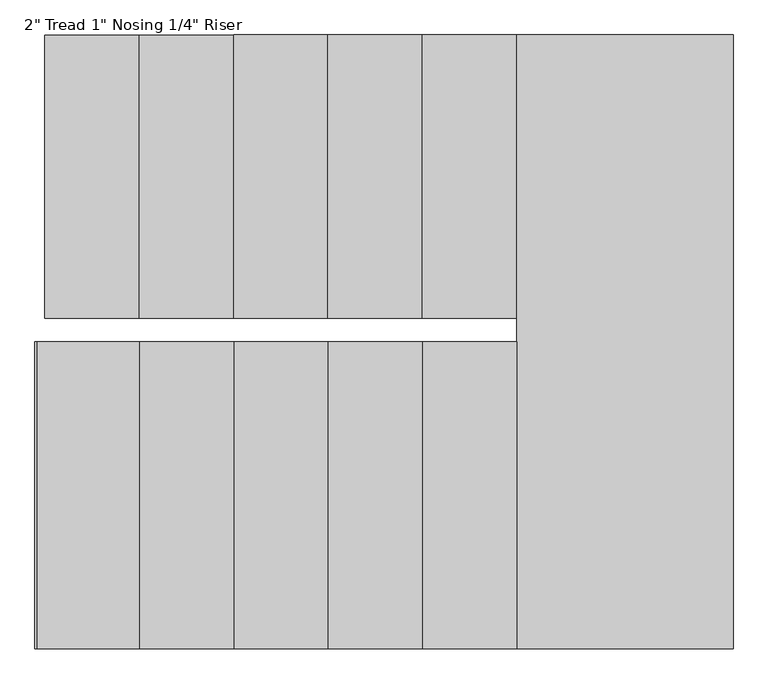
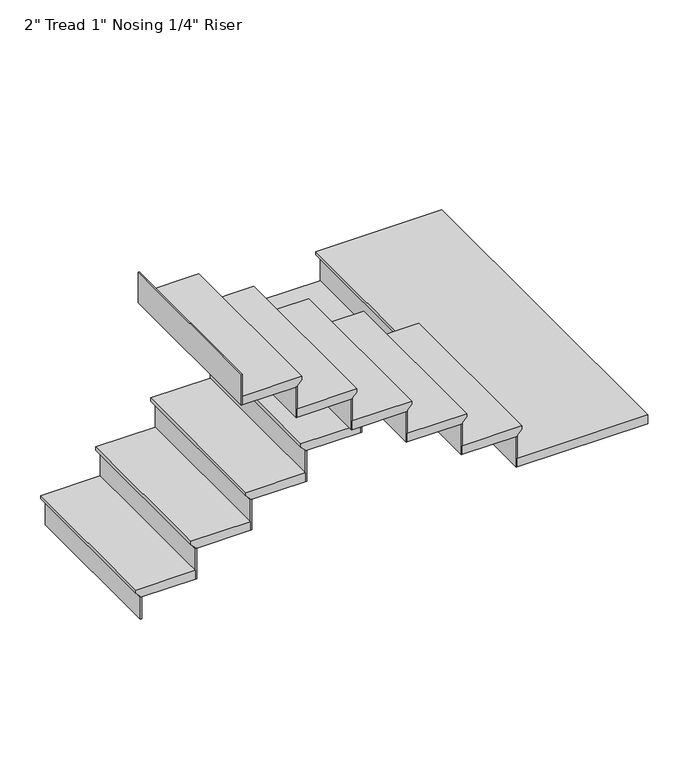
"""IFC4 building model written with IfcOpenShell, lengths in millimetres: stair flight geometry."""

from ifc_helpers import new_model, si_unit, origin, place, context, project, spatial, faceted_brep, source, transform, mapped, element, save


def stair_flight_ab8743af(model_context):
    return source(origin(), model_context, "Body", "Brep", [
        faceted_brep([(-1179.0415084, -2827.3064015, 160.2441176), (-1179.0415084, -2827.3064015, 179.2941176), (-1179.0415084, -1912.9064015, 179.2941176), (-1179.0415084, -1912.9064015, 160.2441176), (-1153.6415084, -2827.3064015, 134.8441176), (-1153.6415084, -1912.9064015, 134.8441176), (-848.8415084, -2827.3064015, 179.2941176), (-848.8415084, -1912.9064015, 179.2941176), (-1153.6415084, -1912.9064015, 128.4941176), (-848.8415084, -1912.9064015, 128.4941176), (-848.8415084, -2827.3064015, 128.4941176), (-1153.6415084, -2827.3064015, 128.4941176)], [[[0, 1, 2, 3]], [[4, 0, 3, 5]], [[2, 1, 6, 7]], [[8, 9, 10, 11]], [[2, 7, 9, 8, 5, 3]], [[8, 11, 4, 5]], [[6, 1, 0, 4, 11, 10]], [[7, 6, 10, 9]]]),
        faceted_brep([(-1153.6415084, -2827.3064015, 128.4941176), (-1153.6415084, -2827.3064015, 0.0), (-1147.2915084, -2827.3064015, 0.0), (-1147.2915084, -2827.3064015, 128.4941176), (-1153.6415084, -1912.9064015, 128.4941176), (-1147.2915084, -1912.9064015, 128.4941176), (-1147.2915084, -1912.9064015, 0.0), (-1153.6415084, -1912.9064015, 0.0)], [[[0, 1, 2, 3]], [[4, 5, 6, 7]], [[1, 0, 4, 7]], [[2, 1, 7, 6]], [[3, 2, 6, 5]], [[0, 3, 5, 4]]]),
        faceted_brep([(-848.8415084, -2827.3064015, 307.7882353), (-848.8415084, -2827.3064015, 128.4941176), (-842.4915084, -2827.3064015, 128.4941176), (-842.4915084, -2827.3064015, 307.7882353), (-848.8415084, -1912.9064015, 307.7882353), (-842.4915084, -1912.9064015, 307.7882353), (-842.4915084, -1912.9064015, 128.4941176), (-848.8415084, -1912.9064015, 128.4941176)], [[[0, 1, 2, 3]], [[4, 5, 6, 7]], [[1, 0, 4, 7]], [[2, 1, 7, 6]], [[3, 2, 6, 5]], [[0, 3, 5, 4]]]),
        faceted_brep([(-874.2415084, -1912.9064015, 358.5882353), (-874.2415084, -2827.3064015, 358.5882353), (-544.0415084, -2827.3064015, 358.5882353), (-544.0415084, -1912.9064015, 358.5882353), (-848.8415084, -1912.9064015, 307.7882353), (-544.0415084, -1912.9064015, 307.7882353), (-544.0415084, -2827.3064015, 307.7882353), (-848.8415084, -2827.3064015, 307.7882353), (-848.8415084, -1912.9064015, 314.1382353), (-874.2415084, -1912.9064015, 339.5382353), (-848.8415084, -2827.3064015, 314.1382353), (-874.2415084, -2827.3064015, 339.5382353)], [[[0, 1, 2, 3]], [[4, 5, 6, 7]], [[0, 3, 5, 4, 8, 9]], [[4, 7, 10, 8]], [[2, 1, 11, 10, 7, 6]], [[3, 2, 6, 5]], [[11, 1, 0, 9]], [[10, 11, 9, 8]]]),
        faceted_brep([(-544.0415084, -2827.3064015, 487.0823529), (-544.0415084, -2827.3064015, 307.7882353), (-537.6915084, -2827.3064015, 307.7882353), (-537.6915084, -2827.3064015, 487.0823529), (-544.0415084, -1912.9064015, 487.0823529), (-537.6915084, -1912.9064015, 487.0823529), (-537.6915084, -1912.9064015, 307.7882353), (-544.0415084, -1912.9064015, 307.7882353)], [[[0, 1, 2, 3]], [[4, 5, 6, 7]], [[1, 0, 4, 7]], [[2, 1, 7, 6]], [[3, 2, 6, 5]], [[0, 3, 5, 4]]]),
        faceted_brep([(-569.4415084, -1912.9064015, 537.8823529), (-569.4415084, -2827.3064015, 537.8823529), (-239.2415084, -2827.3064015, 537.8823529), (-239.2415084, -1912.9064015, 537.8823529), (-544.0415084, -1912.9064015, 487.0823529), (-239.2415084, -1912.9064015, 487.0823529), (-239.2415084, -2827.3064015, 487.0823529), (-544.0415084, -2827.3064015, 487.0823529), (-544.0415084, -1912.9064015, 493.4323529), (-569.4415084, -1912.9064015, 518.8323529), (-544.0415084, -2827.3064015, 493.4323529), (-569.4415084, -2827.3064015, 518.8323529)], [[[0, 1, 2, 3]], [[4, 5, 6, 7]], [[0, 3, 5, 4, 8, 9]], [[4, 7, 10, 8]], [[2, 1, 11, 10, 7, 6]], [[3, 2, 6, 5]], [[11, 1, 0, 9]], [[10, 11, 9, 8]]]),
        faceted_brep([(-239.2415084, -2827.3064015, 666.3764706), (-239.2415084, -2827.3064015, 487.0823529), (-232.8915084, -2827.3064015, 487.0823529), (-232.8915084, -2827.3064015, 666.3764706), (-239.2415084, -1912.9064015, 666.3764706), (-232.8915084, -1912.9064015, 666.3764706), (-232.8915084, -1912.9064015, 487.0823529), (-239.2415084, -1912.9064015, 487.0823529)], [[[0, 1, 2, 3]], [[4, 5, 6, 7]], [[1, 0, 4, 7]], [[2, 1, 7, 6]], [[3, 2, 6, 5]], [[0, 3, 5, 4]]]),
        faceted_brep([(-264.6415084, -1912.9064015, 717.1764706), (-264.6415084, -2827.3064015, 717.1764706), (65.5584916, -2827.3064015, 717.1764706), (65.5584916, -1912.9064015, 717.1764706), (-239.2415084, -1912.9064015, 666.3764706), (65.5584916, -1912.9064015, 666.3764706), (65.5584916, -2827.3064015, 666.3764706), (-239.2415084, -2827.3064015, 666.3764706), (-239.2415084, -1912.9064015, 672.7264706), (-264.6415084, -1912.9064015, 698.1264706), (-239.2415084, -2827.3064015, 672.7264706), (-264.6415084, -2827.3064015, 698.1264706)], [[[0, 1, 2, 3]], [[4, 5, 6, 7]], [[0, 3, 5, 4, 8, 9]], [[4, 7, 10, 8]], [[2, 1, 11, 10, 7, 6]], [[3, 2, 6, 5]], [[11, 1, 0, 9]], [[10, 11, 9, 8]]]),
        faceted_brep([(65.5584916, -2827.3064015, 845.6705882), (65.5584916, -2827.3064015, 666.3764706), (71.9084916, -2827.3064015, 666.3764706), (71.9084916, -2827.3064015, 845.6705882), (65.5584916, -1912.9064015, 845.6705882), (71.9084916, -1912.9064015, 845.6705882), (71.9084916, -1912.9064015, 666.3764706), (65.5584916, -1912.9064015, 666.3764706)], [[[0, 1, 2, 3]], [[4, 5, 6, 7]], [[1, 0, 4, 7]], [[2, 1, 7, 6]], [[3, 2, 6, 5]], [[0, 3, 5, 4]]]),
        faceted_brep([(40.1584916, -1912.9064015, 896.4705882), (40.1584916, -2827.3064015, 896.4705882), (370.3584916, -2827.3064015, 896.4705882), (370.3584916, -1912.9064015, 896.4705882), (65.5584916, -1912.9064015, 845.6705882), (370.3584916, -1912.9064015, 845.6705882), (370.3584916, -2827.3064015, 845.6705882), (65.5584916, -2827.3064015, 845.6705882), (65.5584916, -1912.9064015, 852.0205882), (40.1584916, -1912.9064015, 877.4205882), (65.5584916, -2827.3064015, 852.0205882), (40.1584916, -2827.3064015, 877.4205882)], [[[0, 1, 2, 3]], [[4, 5, 6, 7]], [[0, 3, 5, 4, 8, 9]], [[4, 7, 10, 8]], [[2, 1, 11, 10, 7, 6]], [[3, 2, 6, 5]], [[11, 1, 0, 9]], [[10, 11, 9, 8]]]),
        faceted_brep([(370.3584916, -2827.3064015, 1024.9647059), (370.3584916, -2827.3064015, 845.6705882), (376.7084916, -2827.3064015, 845.6705882), (376.7084916, -2827.3064015, 1024.9647059), (370.3584916, -1912.9064015, 1024.9647059), (376.7084916, -1912.9064015, 1024.9647059), (376.7084916, -1912.9064015, 845.6705882), (370.3584916, -1912.9064015, 845.6705882)], [[[0, 1, 2, 3]], [[4, 5, 6, 7]], [[1, 0, 4, 7]], [[2, 1, 7, 6]], [[3, 2, 6, 5]], [[0, 3, 5, 4]]]),
        faceted_brep([(319.5584916, -3894.1064015, 1075.7647059), (1043.4584916, -3894.1064015, 1075.7647059), (1043.4584916, -1912.9064015, 1075.7647059), (344.9584916, -1912.9064015, 1075.7647059), (344.9584916, -2903.5064015, 1075.7647059), (319.5584916, -2903.5064015, 1075.7647059), (1043.4584916, -3894.1064015, 1024.9647059), (319.5584916, -3894.1064015, 1024.9647059), (319.5584916, -2903.5064015, 1024.9647059), (344.9584916, -2903.5064015, 1024.9647059), (344.9584916, -2827.3064015, 1024.9647059), (370.3584916, -2827.3064015, 1024.9647059), (370.3584916, -1912.9064015, 1024.9647059), (1043.4584916, -1912.9064015, 1024.9647059), (370.3584916, -1912.9064015, 1031.3147059), (344.9584916, -1912.9064015, 1056.7147059), (370.3584916, -2827.3064015, 1031.3147059), (344.9584916, -2827.3064015, 1056.7147059)], [[[0, 1, 2, 3, 4, 5]], [[6, 7, 8, 9, 10, 11, 12, 13]], [[1, 0, 7, 6]], [[2, 1, 6, 13]], [[3, 2, 13, 12, 14, 15]], [[12, 11, 16, 14]], [[11, 10, 17, 16]], [[4, 3, 15, 17, 10, 9]], [[5, 4, 9, 8]], [[0, 5, 8, 7]], [[15, 14, 16, 17]]]),
        faceted_brep([(319.5584916, -2903.5064015, 1204.2588235), (319.5584916, -2903.5064015, 1024.9647059), (313.2084916, -2903.5064015, 1024.9647059), (313.2084916, -2903.5064015, 1204.2588235), (319.5584916, -3894.1064015, 1204.2588235), (313.2084916, -3894.1064015, 1204.2588235), (313.2084916, -3894.1064015, 1024.9647059), (319.5584916, -3894.1064015, 1024.9647059)], [[[0, 1, 2, 3]], [[4, 5, 6, 7]], [[1, 0, 4, 7]], [[2, 1, 7, 6]], [[3, 2, 6, 5]], [[0, 3, 5, 4]]]),
        faceted_brep([(344.9584916, -3894.1064015, 1255.0588235), (344.9584916, -2903.5064015, 1255.0588235), (14.7584916, -2903.5064015, 1255.0588235), (14.7584916, -3894.1064015, 1255.0588235), (319.5584916, -3894.1064015, 1204.2588235), (14.7584916, -3894.1064015, 1204.2588235), (14.7584916, -2903.5064015, 1204.2588235), (319.5584916, -2903.5064015, 1204.2588235), (319.5584916, -3894.1064015, 1210.6088235), (344.9584916, -3894.1064015, 1236.0088235), (319.5584916, -2903.5064015, 1210.6088235), (344.9584916, -2903.5064015, 1236.0088235)], [[[0, 1, 2, 3]], [[4, 5, 6, 7]], [[0, 3, 5, 4, 8, 9]], [[4, 7, 10, 8]], [[2, 1, 11, 10, 7, 6]], [[3, 2, 6, 5]], [[11, 1, 0, 9]], [[10, 11, 9, 8]]]),
        faceted_brep([(14.7584916, -2903.5064015, 1383.5529412), (14.7584916, -2903.5064015, 1204.2588235), (8.4084916, -2903.5064015, 1204.2588235), (8.4084916, -2903.5064015, 1383.5529412), (14.7584916, -3894.1064015, 1383.5529412), (8.4084916, -3894.1064015, 1383.5529412), (8.4084916, -3894.1064015, 1204.2588235), (14.7584916, -3894.1064015, 1204.2588235)], [[[0, 1, 2, 3]], [[4, 5, 6, 7]], [[1, 0, 4, 7]], [[2, 1, 7, 6]], [[3, 2, 6, 5]], [[0, 3, 5, 4]]]),
        faceted_brep([(40.1584916, -3894.1064015, 1434.3529412), (40.1584916, -2903.5064015, 1434.3529412), (-290.0415084, -2903.5064015, 1434.3529412), (-290.0415084, -3894.1064015, 1434.3529412), (14.7584916, -3894.1064015, 1383.5529412), (-290.0415084, -3894.1064015, 1383.5529412), (-290.0415084, -2903.5064015, 1383.5529412), (14.7584916, -2903.5064015, 1383.5529412), (14.7584916, -3894.1064015, 1389.9029412), (40.1584916, -3894.1064015, 1415.3029412), (14.7584916, -2903.5064015, 1389.9029412), (40.1584916, -2903.5064015, 1415.3029412)], [[[0, 1, 2, 3]], [[4, 5, 6, 7]], [[0, 3, 5, 4, 8, 9]], [[4, 7, 10, 8]], [[2, 1, 11, 10, 7, 6]], [[3, 2, 6, 5]], [[11, 1, 0, 9]], [[10, 11, 9, 8]]]),
        faceted_brep([(-290.0415084, -2903.5064015, 1562.8470588), (-290.0415084, -2903.5064015, 1383.5529412), (-296.3915084, -2903.5064015, 1383.5529412), (-296.3915084, -2903.5064015, 1562.8470588), (-290.0415084, -3894.1064015, 1562.8470588), (-296.3915084, -3894.1064015, 1562.8470588), (-296.3915084, -3894.1064015, 1383.5529412), (-290.0415084, -3894.1064015, 1383.5529412)], [[[0, 1, 2, 3]], [[4, 5, 6, 7]], [[1, 0, 4, 7]], [[2, 1, 7, 6]], [[3, 2, 6, 5]], [[0, 3, 5, 4]]]),
        faceted_brep([(-264.6415084, -3894.1064015, 1613.6470588), (-264.6415084, -2903.5064015, 1613.6470588), (-594.8415084, -2903.5064015, 1613.6470588), (-594.8415084, -3894.1064015, 1613.6470588), (-290.0415084, -3894.1064015, 1562.8470588), (-594.8415084, -3894.1064015, 1562.8470588), (-594.8415084, -2903.5064015, 1562.8470588), (-290.0415084, -2903.5064015, 1562.8470588), (-290.0415084, -3894.1064015, 1569.1970588), (-264.6415084, -3894.1064015, 1594.5970588), (-290.0415084, -2903.5064015, 1569.1970588), (-264.6415084, -2903.5064015, 1594.5970588)], [[[0, 1, 2, 3]], [[4, 5, 6, 7]], [[0, 3, 5, 4, 8, 9]], [[4, 7, 10, 8]], [[2, 1, 11, 10, 7, 6]], [[3, 2, 6, 5]], [[11, 1, 0, 9]], [[10, 11, 9, 8]]]),
        faceted_brep([(-594.8415084, -2903.5064015, 1742.1411765), (-594.8415084, -2903.5064015, 1562.8470588), (-601.1915084, -2903.5064015, 1562.8470588), (-601.1915084, -2903.5064015, 1742.1411765), (-594.8415084, -3894.1064015, 1742.1411765), (-601.1915084, -3894.1064015, 1742.1411765), (-601.1915084, -3894.1064015, 1562.8470588), (-594.8415084, -3894.1064015, 1562.8470588)], [[[0, 1, 2, 3]], [[4, 5, 6, 7]], [[1, 0, 4, 7]], [[2, 1, 7, 6]], [[3, 2, 6, 5]], [[0, 3, 5, 4]]]),
        faceted_brep([(-569.4415084, -3894.1064015, 1792.9411765), (-569.4415084, -2903.5064015, 1792.9411765), (-899.6415084, -2903.5064015, 1792.9411765), (-899.6415084, -3894.1064015, 1792.9411765), (-594.8415084, -3894.1064015, 1742.1411765), (-899.6415084, -3894.1064015, 1742.1411765), (-899.6415084, -2903.5064015, 1742.1411765), (-594.8415084, -2903.5064015, 1742.1411765), (-594.8415084, -3894.1064015, 1748.4911765), (-569.4415084, -3894.1064015, 1773.8911765), (-594.8415084, -2903.5064015, 1748.4911765), (-569.4415084, -2903.5064015, 1773.8911765)], [[[0, 1, 2, 3]], [[4, 5, 6, 7]], [[0, 3, 5, 4, 8, 9]], [[4, 7, 10, 8]], [[2, 1, 11, 10, 7, 6]], [[3, 2, 6, 5]], [[11, 1, 0, 9]], [[10, 11, 9, 8]]]),
        faceted_brep([(-899.6415084, -2903.5064015, 1921.4352941), (-899.6415084, -2903.5064015, 1742.1411765), (-905.9915084, -2903.5064015, 1742.1411765), (-905.9915084, -2903.5064015, 1921.4352941), (-899.6415084, -3894.1064015, 1921.4352941), (-905.9915084, -3894.1064015, 1921.4352941), (-905.9915084, -3894.1064015, 1742.1411765), (-899.6415084, -3894.1064015, 1742.1411765)], [[[0, 1, 2, 3]], [[4, 5, 6, 7]], [[1, 0, 4, 7]], [[2, 1, 7, 6]], [[3, 2, 6, 5]], [[0, 3, 5, 4]]]),
        faceted_brep([(-1204.4415084, -2903.5064015, 2100.7294118), (-1204.4415084, -2903.5064015, 1921.4352941), (-1210.7915084, -2903.5064015, 1921.4352941), (-1210.7915084, -2903.5064015, 2100.7294118), (-1204.4415084, -3894.1064015, 2100.7294118), (-1210.7915084, -3894.1064015, 2100.7294118), (-1210.7915084, -3894.1064015, 1921.4352941), (-1204.4415084, -3894.1064015, 1921.4352941)], [[[0, 1, 2, 3]], [[4, 5, 6, 7]], [[1, 0, 4, 7]], [[2, 1, 7, 6]], [[3, 2, 6, 5]], [[0, 3, 5, 4]]]),
        faceted_brep([(-874.2415084, -3894.1064015, 1972.2352941), (-874.2415084, -2903.5064015, 1972.2352941), (-1204.4415084, -2903.5064015, 1972.2352941), (-1204.4415084, -3894.1064015, 1972.2352941), (-899.6415084, -3894.1064015, 1921.4352941), (-1204.4415084, -3894.1064015, 1921.4352941), (-1204.4415084, -2903.5064015, 1921.4352941), (-899.6415084, -2903.5064015, 1921.4352941), (-899.6415084, -3894.1064015, 1927.7852941), (-874.2415084, -3894.1064015, 1953.1852941), (-899.6415084, -2903.5064015, 1927.7852941), (-874.2415084, -2903.5064015, 1953.1852941)], [[[0, 1, 2, 3]], [[4, 5, 6, 7]], [[0, 3, 5, 4, 8, 9]], [[4, 7, 10, 8]], [[2, 1, 11, 10, 7, 6]], [[3, 2, 6, 5]], [[11, 1, 0, 9]], [[10, 11, 9, 8]]]),
    ])


if __name__ == "__main__":
    model = new_model("IFC4")
    model_context = context("Model", 3, world=origin())
    ifc_project = project(units=[si_unit("LENGTHUNIT", "METRE", prefix="MILLI")], contexts=[model_context])
    site = spatial("IfcSite", under=ifc_project)
    building = spatial("IfcBuilding", under=site)
    placement = place(None, origin())
    stair_flight_shape = stair_flight_ab8743af(model_context)
    element("IfcStairFlight", 1, ObjectType="2\" Tread 1\" Nosing 1/4\" Riser", at=placement, inside=building, context=model_context, shape_type="MappedRepresentation", body=[
        mapped(stair_flight_shape, transform((0.0, 0.0, 0.0), x_axis=(1.0, 0.0, 0.0), y_axis=(0.0, 1.0, 0.0), z_axis=(0.0, 0.0, 1.0))),
    ])
    save(model, "model.ifc")
